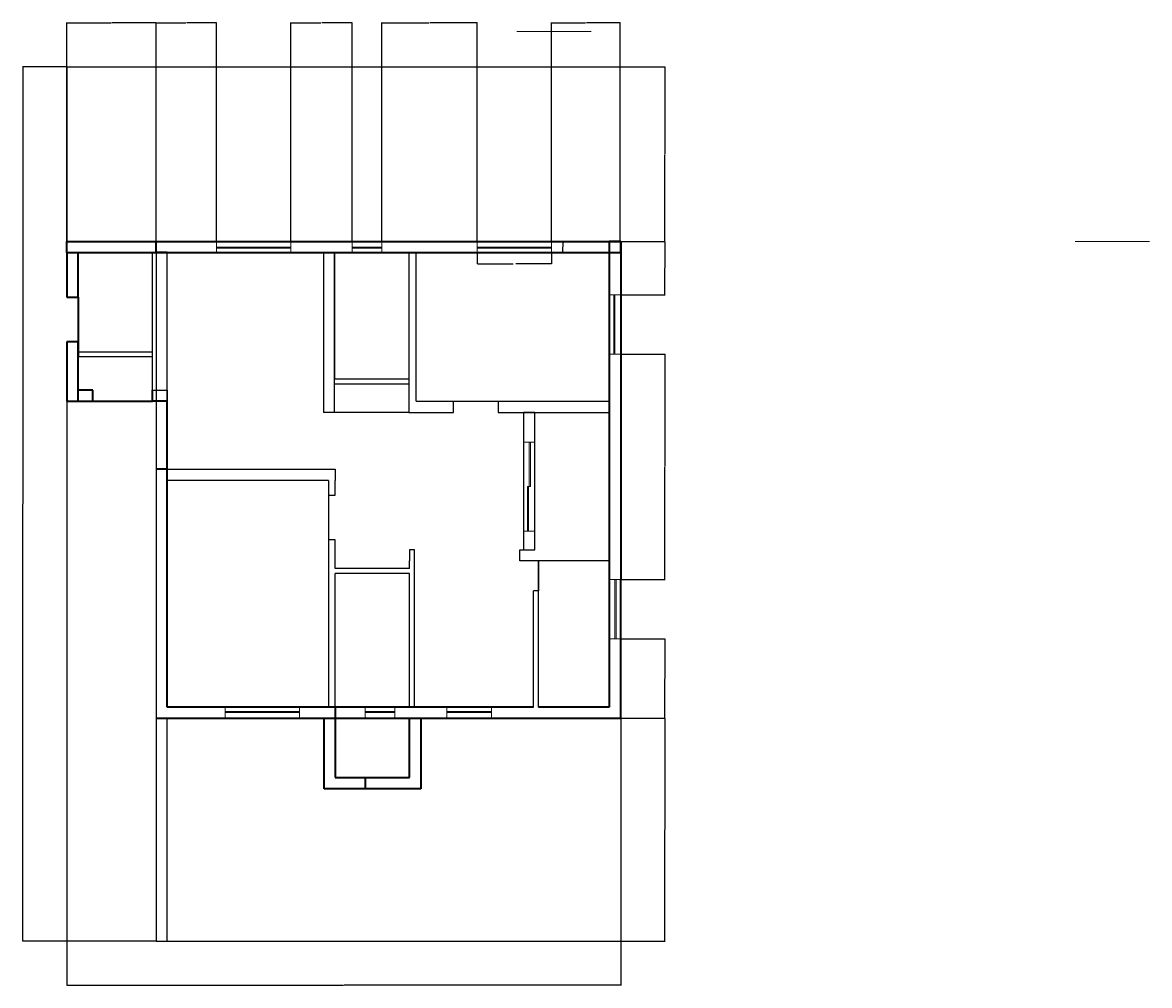
# Model space of a CAD drawing. Units: inches. Extents: x 2029 to 8798, y 1998 to 6373.
# Tile 11 of 11: x 7888 to 8798, y 1998 to 2776. Entities that reach past the tile are written whole.
import ezdxf

# ---------------------------------------------------------------- set-up
doc = ezdxf.new("R2010")
doc.units = ezdxf.units.IN
for name, color, linetype, lineweight in [('A-ANNO-DIMS', 2, 'Continuous', 18), ('A-GENM-REFR', 8, 'Continuous', 13), ('A-GLAZ', 4, 'Continuous', 18), ('A-WALL-CIRC', 7, 'Continuous', 25), ('A-WALL-EXTR', 7, 'Continuous', 35), ('A-WALL-INTR', 7, 'Continuous', 25)]:
    doc.layers.add(name, color=color, linetype=linetype, lineweight=lineweight)
doc.styles.get("Standard").update_dxf_attribs({"font": 'arial.ttf'})
doc.dimstyles.get("Standard").update_dxf_attribs({"dimtxt": 0.18, "dimasz": 0.18, "dimexe": 0.18, "dimexo": 0.0625, "dimgap": 0.09, "dimtad": 0, "dimtih": 1, "dimtoh": 1, "dimdec": 4, "dimzin": 0, "dimdsep": 46, "dimtxsty": 'Standard', "dimcen": 0.09, "dimadec": 0, "dimazin": 0, "dimtfac": 1, "dimtdec": 4, "dimtofl": 0, "dimtmove": 0, "dimatfit": 3, "dimfxl": 1, "dimtolj": 1, "dimtzin": 0, "dimarcsym": 0})

# ---------------------------------------------------------------- blocks, each defined once
blk = doc.blocks.new('WIN-60')
for p, q in [((0, 0), (0, 9)), ((0, 4.5), (60, 4.5)), ((0, 3.5), (60, 3.5)), ((60, 9), (60, 0))]:
    blk.add_line(p, q)
blk = doc.blocks.new('WIN-36')
for p, q in [((0, 36), (9, 36)), ((3.5, 36), (3.5, 0)), ((4.5, 36), (4.5, 0)), ((9, 0), (0, 0))]:
    blk.add_line(p, q)
blk = doc.blocks.new('WIN-24')
for p, q in [((0, 0), (0, 9)), ((0, 4.5), (24, 4.5)), ((0, 3.5), (24, 3.5)), ((24, 9), (24, 0))]:
    blk.add_line(p, q)
blk = doc.blocks.new('WIN-48-DEEP-JAMB')
for p, q in [((9.38, 48), (0, 48)), ((0, 48), (0, 0)), ((3.69, 48), (3.69, 0)), ((4.69, 48), (4.69, 0)), ((0, 0), (9.38, 0))]:
    blk.add_line(p, q)
blk = doc.blocks.new('GLAZ-SLIDER-72-V')
for p, q in [((0, 72), (9, 72)), ((4.5, 72), (4.5, 36)), ((5.5, 72), (5.5, 36)), ((9, 72), (9, 0)), ((3, 36), (3, 0)), ((3, 36), (4, 36)), ((4, 36), (4, 0)), ((4.5, 36), (5.5, 36)), ((9, 0), (0, 0))]:
    blk.add_line(p, q)
blk = doc.blocks.new('*D13')
at = {"layer": 'A-ANNO-DIMS', "color": 0, "lineweight": -2, "transparency": 16777216}
for p, q in [((8255.56, 2590.18), (8255.56, 2581.07)), ((8315.56, 2590.18), (8315.56, 2581.07)), ((8255.74, 2581.25), (8284.44, 2581.25)), ((8315.38, 2581.25), (8286.67, 2581.25))]:
    blk.add_line(p, q, dxfattribs=at)
at = {"layer": 'A-ANNO-DIMS', "color": 0, "transparency": 16777216}
for points in [[(8255.74, 2581.28), (8255.74, 2581.22), (8255.56, 2581.25)], [(8315.38, 2581.28), (8315.38, 2581.22), (8315.56, 2581.25)]]:
    blk.add_solid(points, dxfattribs=at)
at = {"layer": 'Defpoints', "color": 0, "transparency": 16777216}
for p in [(8255.56, 2590.25), (8315.56, 2590.25), (8315.56, 2581.25)]:
    blk.add_point(p, dxfattribs=at)
at = {"layer": 'A-ANNO-DIMS', "color": 0, "transparency": 16777216, "insert": (8285.56, 2581.25), "char_height": 0.18, "attachment_point": 5}
blk.add_mtext('\\A1;WINDOW 60 TYP.', dxfattribs=at)
blk = doc.blocks.new('*D14')
at = {"layer": 'A-ANNO-DIMS', "color": 0, "lineweight": -2, "transparency": 16777216}
for p, q in [((8315.62, 2599.25), (8324.74, 2599.25)), ((8324.56, 2599.07), (8324.56, 2594.93)), ((8324.56, 2590.43), (8324.56, 2594.57)), ((8315.62, 2590.25), (8324.74, 2590.25))]:
    blk.add_line(p, q, dxfattribs=at)
at = {"layer": 'A-ANNO-DIMS', "color": 0, "transparency": 16777216}
for points in [[(8324.53, 2599.07), (8324.59, 2599.07), (8324.56, 2599.25)], [(8324.53, 2590.43), (8324.59, 2590.43), (8324.56, 2590.25)]]:
    blk.add_solid(points, dxfattribs=at)
at = {"layer": 'Defpoints', "color": 0, "transparency": 16777216}
for p in [(8315.56, 2599.25), (8324.56, 2599.25), (8315.56, 2590.25)]:
    blk.add_point(p, dxfattribs=at)
at = {"layer": 'A-ANNO-DIMS', "color": 0, "transparency": 16777216, "insert": (8324.56, 2594.75), "char_height": 0.18, "attachment_point": 5}
blk.add_mtext('\\A1;9 TYP.', dxfattribs=at)
blk = doc.blocks.new('*D93')
at = {"layer": 'A-ANNO-DIMS', "color": 0, "lineweight": -2, "transparency": 16777216}
for p, q in [((7924.34, 2470.18), (7924.34, 1998.42)), ((8371.34, 2214.18), (8371.34, 1998.42)), ((7924.52, 1998.6), (8147.55, 1998.6)), ((8371.16, 1998.6), (8148.13, 1998.6))]:
    blk.add_line(p, q, dxfattribs=at)
at = {"layer": 'A-ANNO-DIMS', "color": 0, "transparency": 16777216}
for points in [[(7924.52, 1998.63), (7924.52, 1998.57), (7924.34, 1998.6)], [(8371.16, 1998.63), (8371.16, 1998.57), (8371.34, 1998.6)]]:
    blk.add_solid(points, dxfattribs=at)
at = {"layer": 'Defpoints', "color": 0, "transparency": 16777216}
for p in [(7924.34, 2470.25), (8371.34, 2214.25), (8371.34, 1998.6)]:
    blk.add_point(p, dxfattribs=at)
at = {"layer": 'A-ANNO-DIMS', "color": 0, "transparency": 16777216, "insert": (8147.84, 1998.6), "char_height": 0.18, "attachment_point": 5}
blk.add_mtext('\\A1;447', dxfattribs=at)
blk = doc.blocks.new('*D94')
at = {"layer": 'A-ANNO-DIMS', "color": 0, "lineweight": -2, "transparency": 16777216}
for p, q in [((7924.28, 2740.25), (7888.51, 2740.25)), ((7888.69, 2740.07), (7888.69, 2387.43)), ((7888.69, 2034.43), (7888.69, 2387.07)), ((7996.28, 2034.25), (7888.51, 2034.25))]:
    blk.add_line(p, q, dxfattribs=at)
at = {"layer": 'A-ANNO-DIMS', "color": 0, "transparency": 16777216}
for points in [[(7888.66, 2740.07), (7888.72, 2740.07), (7888.69, 2740.25)], [(7888.66, 2034.43), (7888.72, 2034.43), (7888.69, 2034.25)]]:
    blk.add_solid(points, dxfattribs=at)
at = {"layer": 'Defpoints', "color": 0, "transparency": 16777216}
for p in [(7924.34, 2740.25), (7888.69, 2034.25), (7996.34, 2034.25)]:
    blk.add_point(p, dxfattribs=at)
at = {"layer": 'A-ANNO-DIMS', "color": 0, "transparency": 16777216, "insert": (7888.69, 2387.25), "char_height": 0.18, "attachment_point": 5}
blk.add_mtext('\\A1;706', dxfattribs=at)
blk = doc.blocks.new('*D95')
at = {"layer": 'A-ANNO-DIMS', "color": 0, "lineweight": -2, "transparency": 16777216}
for p, q in [((7924.34, 2599.31), (7924.34, 2776.08)), ((7924.52, 2775.9), (7960.12, 2775.9)), ((7996.16, 2775.9), (7960.56, 2775.9)), ((7996.34, 2599.31), (7996.34, 2776.08))]:
    blk.add_line(p, q, dxfattribs=at)
at = {"layer": 'A-ANNO-DIMS', "color": 0, "transparency": 16777216}
for points in [[(7924.52, 2775.93), (7924.52, 2775.87), (7924.34, 2775.9)], [(7996.16, 2775.93), (7996.16, 2775.87), (7996.34, 2775.9)]]:
    blk.add_solid(points, dxfattribs=at)
at = {"layer": 'Defpoints', "color": 0, "transparency": 16777216}
for p in [(7996.34, 2775.9), (7924.34, 2599.25), (7996.34, 2599.25)]:
    blk.add_point(p, dxfattribs=at)
at = {"layer": 'A-ANNO-DIMS', "color": 0, "transparency": 16777216, "insert": (7960.34, 2775.9), "char_height": 0.18, "attachment_point": 5}
blk.add_mtext('\\A1;72', dxfattribs=at)
blk = doc.blocks.new('*D96')
at = {"layer": 'A-ANNO-DIMS', "color": 0, "lineweight": -2, "transparency": 16777216}
for p, q in [((7996.34, 2599.31), (7996.34, 2776.08)), ((7996.52, 2775.9), (8020.25, 2775.9)), ((8044.78, 2775.9), (8021.05, 2775.9)), ((8044.96, 2599.31), (8044.96, 2776.08))]:
    blk.add_line(p, q, dxfattribs=at)
at = {"layer": 'A-ANNO-DIMS', "color": 0, "transparency": 16777216}
for points in [[(7996.52, 2775.93), (7996.52, 2775.87), (7996.34, 2775.9)], [(8044.78, 2775.93), (8044.78, 2775.87), (8044.96, 2775.9)]]:
    blk.add_solid(points, dxfattribs=at)
at = {"layer": 'Defpoints', "color": 0, "transparency": 16777216}
for p in [(8044.96, 2775.9), (7996.34, 2599.25), (8044.96, 2599.25)]:
    blk.add_point(p, dxfattribs=at)
at = {"layer": 'A-ANNO-DIMS', "color": 0, "transparency": 16777216, "insert": (8020.65, 2775.9), "char_height": 0.18, "attachment_point": 5}
blk.add_mtext('\\A1;48.62', dxfattribs=at)
blk = doc.blocks.new('*D97')
at = {"layer": 'A-ANNO-DIMS', "color": 0, "lineweight": -2, "transparency": 16777216}
for p, q in [((8104.96, 2599.31), (8104.96, 2776.08)), ((8105.14, 2775.9), (8129.39, 2775.9)), ((8154.43, 2775.9), (8130.18, 2775.9)), ((8154.61, 2599.31), (8154.61, 2776.08))]:
    blk.add_line(p, q, dxfattribs=at)
at = {"layer": 'A-ANNO-DIMS', "color": 0, "transparency": 16777216}
for points in [[(8105.14, 2775.93), (8105.14, 2775.87), (8104.96, 2775.9)], [(8154.43, 2775.93), (8154.43, 2775.87), (8154.61, 2775.9)]]:
    blk.add_solid(points, dxfattribs=at)
at = {"layer": 'Defpoints', "color": 0, "transparency": 16777216}
for p in [(8154.61, 2775.9), (8104.96, 2599.25), (8154.61, 2599.25)]:
    blk.add_point(p, dxfattribs=at)
at = {"layer": 'A-ANNO-DIMS', "color": 0, "transparency": 16777216, "insert": (8129.78, 2775.9), "char_height": 0.18, "attachment_point": 5}
blk.add_mtext('\\A1;49.65', dxfattribs=at)
blk = doc.blocks.new('*D98')
at = {"layer": 'A-ANNO-DIMS', "color": 0, "lineweight": -2, "transparency": 16777216}
for p, q in [((8178.61, 2599.31), (8178.61, 2776.08)), ((8178.79, 2775.9), (8216.69, 2775.9)), ((8255.38, 2775.9), (8217.48, 2775.9)), ((8255.56, 2599.31), (8255.56, 2776.08))]:
    blk.add_line(p, q, dxfattribs=at)
at = {"layer": 'A-ANNO-DIMS', "color": 0, "transparency": 16777216}
for points in [[(8178.79, 2775.93), (8178.79, 2775.87), (8178.61, 2775.9)], [(8255.38, 2775.93), (8255.38, 2775.87), (8255.56, 2775.9)]]:
    blk.add_solid(points, dxfattribs=at)
at = {"layer": 'Defpoints', "color": 0, "transparency": 16777216}
for p in [(8255.56, 2775.9), (8178.61, 2599.25), (8255.56, 2599.25)]:
    blk.add_point(p, dxfattribs=at)
at = {"layer": 'A-ANNO-DIMS', "color": 0, "transparency": 16777216, "insert": (8217.08, 2775.9), "char_height": 0.18, "attachment_point": 5}
blk.add_mtext('\\A1;76.95', dxfattribs=at)
blk = doc.blocks.new('*D99')
at = {"layer": 'A-ANNO-DIMS', "color": 0, "lineweight": -2, "transparency": 16777216}
for p, q in [((8315.56, 2599.31), (8315.56, 2776.08)), ((8315.74, 2775.9), (8342.88, 2775.9)), ((8370.78, 2775.9), (8343.64, 2775.9)), ((8370.96, 2599.31), (8370.96, 2776.08))]:
    blk.add_line(p, q, dxfattribs=at)
at = {"layer": 'A-ANNO-DIMS', "color": 0, "transparency": 16777216}
for points in [[(8315.74, 2775.93), (8315.74, 2775.87), (8315.56, 2775.9)], [(8370.78, 2775.93), (8370.78, 2775.87), (8370.96, 2775.9)]]:
    blk.add_solid(points, dxfattribs=at)
at = {"layer": 'Defpoints', "color": 0, "transparency": 16777216}
for p in [(8370.96, 2775.9), (8315.56, 2599.25), (8370.96, 2599.25)]:
    blk.add_point(p, dxfattribs=at)
at = {"layer": 'A-ANNO-DIMS', "color": 0, "transparency": 16777216, "insert": (8343.26, 2775.9), "char_height": 0.18, "attachment_point": 5}
blk.add_mtext('\\A1;55.41', dxfattribs=at)
blk = doc.blocks.new('*D100')
at = {"layer": 'A-ANNO-DIMS', "color": 0, "lineweight": -2, "transparency": 16777216}
for p, q in [((8371.4, 2214.25), (8407.17, 2214.25)), ((8406.99, 2214.07), (8406.99, 2124.43)), ((8406.99, 2034.43), (8406.99, 2124.07)), ((7996.4, 2034.25), (8407.17, 2034.25))]:
    blk.add_line(p, q, dxfattribs=at)
at = {"layer": 'A-ANNO-DIMS', "color": 0, "transparency": 16777216}
for points in [[(8406.96, 2214.07), (8407.02, 2214.07), (8406.99, 2214.25)], [(8406.96, 2034.43), (8407.02, 2034.43), (8406.99, 2034.25)]]:
    blk.add_solid(points, dxfattribs=at)
at = {"layer": 'Defpoints', "color": 0, "transparency": 16777216}
for p in [(8371.34, 2214.25), (8406.99, 2214.25), (7996.34, 2034.25)]:
    blk.add_point(p, dxfattribs=at)
at = {"layer": 'A-ANNO-DIMS', "color": 0, "transparency": 16777216, "insert": (8406.99, 2124.25), "char_height": 0.18, "attachment_point": 5}
blk.add_mtext('\\A1;180', dxfattribs=at)
blk = doc.blocks.new('*D101')
at = {"layer": 'A-ANNO-DIMS', "color": 0, "lineweight": -2, "transparency": 16777216}
for p, q in [((8371.4, 2278.25), (8407.17, 2278.25)), ((8406.99, 2278.07), (8406.99, 2246.43)), ((8406.99, 2214.43), (8406.99, 2246.07)), ((8371.4, 2214.25), (8407.17, 2214.25))]:
    blk.add_line(p, q, dxfattribs=at)
at = {"layer": 'A-ANNO-DIMS', "color": 0, "transparency": 16777216}
for points in [[(8406.96, 2278.07), (8407.02, 2278.07), (8406.99, 2278.25)], [(8406.96, 2214.43), (8407.02, 2214.43), (8406.99, 2214.25)]]:
    blk.add_solid(points, dxfattribs=at)
at = {"layer": 'Defpoints', "color": 0, "transparency": 16777216}
for p in [(8371.34, 2278.25), (8406.99, 2278.25), (8371.34, 2214.25)]:
    blk.add_point(p, dxfattribs=at)
at = {"layer": 'A-ANNO-DIMS', "color": 0, "transparency": 16777216, "insert": (8406.99, 2246.25), "char_height": 0.18, "attachment_point": 5}
blk.add_mtext('\\A1;64', dxfattribs=at)
blk = doc.blocks.new('*D102')
at = {"layer": 'A-ANNO-DIMS', "color": 0, "lineweight": -2, "transparency": 16777216}
for p, q in [((8371.4, 2508.3), (8407.17, 2508.3)), ((8406.99, 2508.12), (8406.99, 2417.45)), ((8406.99, 2326.43), (8406.99, 2417.09)), ((8371.4, 2326.25), (8407.17, 2326.25))]:
    blk.add_line(p, q, dxfattribs=at)
at = {"layer": 'A-ANNO-DIMS', "color": 0, "transparency": 16777216}
for points in [[(8406.96, 2508.12), (8407.02, 2508.12), (8406.99, 2508.3)], [(8406.96, 2326.43), (8407.02, 2326.43), (8406.99, 2326.25)]]:
    blk.add_solid(points, dxfattribs=at)
at = {"layer": 'Defpoints', "color": 0, "transparency": 16777216}
for p in [(8371.34, 2508.3), (8406.99, 2508.3), (8371.34, 2326.25)]:
    blk.add_point(p, dxfattribs=at)
at = {"layer": 'A-ANNO-DIMS', "color": 0, "transparency": 16777216, "insert": (8406.99, 2417.27), "char_height": 0.18, "attachment_point": 5}
blk.add_mtext('\\A1;182.05', dxfattribs=at)
blk = doc.blocks.new('*D103')
at = {"layer": 'A-ANNO-DIMS', "color": 0, "lineweight": -2, "transparency": 16777216}
for p, q in [((8371.03, 2599.25), (8407.17, 2599.25)), ((8406.99, 2599.07), (8406.99, 2577.95)), ((8406.99, 2556.48), (8406.99, 2577.59)), ((8371.4, 2556.3), (8407.17, 2556.3))]:
    blk.add_line(p, q, dxfattribs=at)
at = {"layer": 'A-ANNO-DIMS', "color": 0, "transparency": 16777216}
for points in [[(8406.96, 2599.07), (8407.02, 2599.07), (8406.99, 2599.25)], [(8406.96, 2556.48), (8407.02, 2556.48), (8406.99, 2556.3)]]:
    blk.add_solid(points, dxfattribs=at)
at = {"layer": 'Defpoints', "color": 0, "transparency": 16777216}
for p in [(8370.96, 2599.25), (8406.99, 2599.25), (8371.34, 2556.3)]:
    blk.add_point(p, dxfattribs=at)
at = {"layer": 'A-ANNO-DIMS', "color": 0, "transparency": 16777216, "insert": (8406.99, 2577.77), "char_height": 0.18, "attachment_point": 5}
blk.add_mtext('\\A1;42.95', dxfattribs=at)
blk = doc.blocks.new('*D104')
at = {"layer": 'A-ANNO-DIMS', "color": 0, "lineweight": -2, "transparency": 16777216}
for p, q in [((7924.4, 2740.25), (8407.17, 2740.25)), ((8406.99, 2740.07), (8406.99, 2669.93)), ((8406.99, 2599.43), (8406.99, 2669.57)), ((7924.4, 2599.25), (8407.17, 2599.25))]:
    blk.add_line(p, q, dxfattribs=at)
at = {"layer": 'A-ANNO-DIMS', "color": 0, "transparency": 16777216}
for points in [[(8406.96, 2740.07), (8407.02, 2740.07), (8406.99, 2740.25)], [(8406.96, 2599.43), (8407.02, 2599.43), (8406.99, 2599.25)]]:
    blk.add_solid(points, dxfattribs=at)
at = {"layer": 'Defpoints', "color": 0, "transparency": 16777216}
for p in [(7924.34, 2740.25), (8406.99, 2740.25), (7924.34, 2599.25)]:
    blk.add_point(p, dxfattribs=at)
at = {"layer": 'A-ANNO-DIMS', "color": 0, "transparency": 16777216, "insert": (8406.99, 2669.75), "char_height": 0.18, "attachment_point": 5}
blk.add_mtext('\\A1;141', dxfattribs=at)

msp = doc.modelspace()

# ---------------------------------------------------------------- linework, layer by layer
at = {"layer": 'A-GENM-REFR'}
for p, q in [((8287.3629, 2768.7471), (8347.3629, 2768.7471)), ((8738.1455, 2599.2471), (8798.1455, 2599.2471))]:
    msp.add_line(p, q, dxfattribs=at)
at = {"layer": 'A-GLAZ'}
for p, q in [((8044.9596, 2599.2471), (8104.9596, 2599.2471)), ((8154.6092, 2599.2471), (8178.6092, 2599.2471)), ((8255.5559, 2599.2471), (8315.5559, 2599.2471)), ((8112.0384, 2214.2471), (8052.0384, 2214.2471)), ((8188.9632, 2214.2471), (8164.9632, 2214.2471)), ((8267.1078, 2214.2471), (8231.1078, 2214.2471))]:
    msp.add_line(p, q, dxfattribs=at)
at = {"layer": 'A-WALL-CIRC'}
for p, q in [((7924.342, 2740.2471), (7924.342, 2590.2471)), ((7996.342, 2214.2471), (7996.342, 2094.2471)), ((8005.342, 2034.2471), (8005.342, 2214.2471)), ((7996.342, 2094.2471), (7996.342, 2034.2471)), ((7996.342, 2034.2471), (8005.342, 2034.2471))]:
    msp.add_line(p, q, dxfattribs=at)
at = {"layer": 'A-WALL-EXTR'}
for p, q in [((7924.342, 2590.2471), (7924.342, 2599.2471)), ((7924.342, 2599.2471), (8370.9632, 2599.2471)), ((7996.342, 2590.2471), (7996.342, 2599.2471)), ((8370.9632, 2599.2471), (8361.9632, 2599.2471)), ((8361.9632, 2599.2471), (8361.9632, 2326.2471)), ((8371.342, 2599.2471), (8369.0749, 2599.2471)), ((8371.342, 2590.2471), (8371.342, 2599.2471)), ((8371.342, 2599.2471), (8371.342, 2326.2471)), ((7924.342, 2590.2471), (7924.342, 2554.2471)), ((7924.342, 2590.2471), (8131.342, 2590.2471)), ((7933.342, 2554.2471), (7933.342, 2590.2471)), ((8005.342, 2590.2471), (7996.342, 2590.2471)), ((8005.342, 2590.2471), (8131.342, 2590.2471)), ((8005.342, 2590.2471), (8044.9596, 2590.2471)), ((8027.842, 2590.2471), (8133.7725, 2590.2471)), ((8131.342, 2590.2471), (8371.342, 2590.2471)), ((8140.342, 2590.2471), (8200.342, 2590.2471)), ((8140.342, 2590.2471), (8154.6092, 2590.2471)), ((8206.342, 2590.2471), (8255.5559, 2590.2471)), ((8371.342, 2590.2471), (8371.342, 2556.2967)), ((7924.342, 2554.2471), (7933.342, 2554.2471)), ((7933.342, 2554.2471), (7933.342, 2518.2471)), ((7933.342, 2518.2471), (7924.342, 2518.2471)), ((7924.342, 2518.2471), (7924.342, 2470.2471)), ((7933.342, 2470.2471), (7933.342, 2518.2471)), ((7933.342, 2518.2471), (7933.342, 2506.2471)), ((7945.342, 2479.2471), (7933.342, 2479.2471)), ((7945.342, 2470.2471), (7945.342, 2479.2471)), ((7993.342, 2470.2471), (7993.342, 2479.2471)), ((7924.342, 2470.2471), (7933.342, 2470.2471)), ((7933.342, 2470.2471), (7945.342, 2470.2471)), ((7945.342, 2470.2471), (7993.342, 2470.2471)), ((8005.342, 2470.2471), (7993.342, 2470.2471)), ((8005.342, 2470.2471), (7993.342, 2470.2471)), ((8005.342, 2223.2471), (8005.342, 2470.2471)), ((8361.9632, 2461.2471), (8361.9632, 2341.2471)), ((8005.342, 2415.2471), (7996.342, 2415.2471)), ((8005.342, 2415.2471), (8005.342, 2415.2471)), ((8005.342, 2406.2471), (8005.342, 2415.2471)), ((8005.342, 2223.2471), (8005.342, 2406.2471)), ((8361.9632, 2341.2471), (8361.9632, 2223.2471)), ((8371.342, 2223.2471), (8371.342, 2326.2471)), ((8298.9632, 2223.2471), (8005.342, 2223.2471)), ((8135.342, 2223.2471), (8112.0384, 2223.2471)), ((8196.9632, 2223.2471), (8136.9632, 2223.2471)), ((8200.9632, 2223.2471), (8140.9632, 2223.2471)), ((8200.9632, 2223.2471), (8140.9632, 2223.2471)), ((8140.9632, 2223.2471), (8140.9632, 2214.2471)), ((8200.9632, 2223.2471), (8188.9632, 2223.2471)), ((8298.9632, 2223.2471), (8202.9632, 2223.2471)), ((8298.9632, 2223.2471), (8267.1078, 2223.2471)), ((8300.9632, 2223.2471), (8298.9632, 2223.2471)), ((8361.9632, 2223.2471), (8304.9632, 2223.2471)), ((8361.9632, 2223.2471), (8304.9632, 2223.2471)), ((8371.342, 2214.2471), (8371.342, 2223.2471)), ((7996.342, 2214.2471), (8371.342, 2214.2471)), ((8131.9632, 2157.2471), (8131.9632, 2214.2471)), ((8140.9632, 2214.2471), (8140.9632, 2166.2471)), ((8200.9632, 2166.2471), (8200.9632, 2214.2471)), ((8200.9632, 2214.2471), (8209.9632, 2214.2471)), ((8209.9632, 2214.2471), (8209.9632, 2157.2471)), ((8140.9632, 2166.2471), (8164.9632, 2166.2471)), ((8164.9632, 2166.2471), (8164.9632, 2157.2471)), ((8164.9632, 2166.2471), (8200.9632, 2166.2471)), ((8140.9632, 2157.2471), (8131.9632, 2157.2471)), ((8164.9632, 2157.2471), (8140.9632, 2157.2471)), ((8209.9632, 2157.2471), (8164.9632, 2157.2471))]:
    msp.add_line(p, q, dxfattribs=at)
at = {"layer": 'A-WALL-INTR'}
for p, q in [((7993.342, 2479.2471), (7993.342, 2590.2471)), ((7996.342, 2590.2471), (7996.342, 2214.2471)), ((8005.342, 2470.2471), (8005.342, 2590.2471)), ((8131.342, 2590.2471), (8131.342, 2461.2471)), ((8140.342, 2461.2471), (8140.342, 2590.2471)), ((8140.342, 2590.2471), (8140.342, 2488.2471)), ((8200.342, 2590.2471), (8200.342, 2470.2471)), ((8206.342, 2470.2471), (8206.342, 2590.2471)), ((7933.342, 2510.2471), (7993.342, 2510.2471)), ((7933.342, 2506.2471), (7993.342, 2506.2471)), ((8140.342, 2488.2471), (8200.342, 2488.2471)), ((8140.342, 2484.2471), (8200.342, 2484.2471)), ((7993.342, 2479.2471), (8005.342, 2479.2471)), ((8005.342, 2479.2471), (8005.342, 2470.2471)), ((8200.342, 2470.2471), (8200.342, 2461.2471)), ((8206.342, 2470.2471), (8361.9632, 2470.2471)), ((8236.342, 2461.2471), (8236.342, 2470.2471)), ((8236.342, 2470.2471), (8272.342, 2470.2471)), ((8272.342, 2470.2471), (8272.342, 2461.2471)), ((8140.342, 2461.2471), (8131.342, 2461.2471)), ((8200.342, 2461.2471), (8140.342, 2461.2471)), ((8200.342, 2461.2471), (8206.342, 2461.2471)), ((8200.342, 2461.2471), (8236.342, 2461.2471)), ((8206.342, 2461.2471), (8236.342, 2461.2471)), ((8272.342, 2461.2471), (8361.9632, 2461.2471)), ((8301.9632, 2461.2471), (8292.9632, 2461.2471)), ((8292.9632, 2461.2471), (8292.9632, 2350.2471)), ((8292.9632, 2461.2471), (8292.9632, 2437.2471)), ((8301.9632, 2350.2471), (8301.9632, 2461.2471)), ((8005.342, 2415.2471), (8140.9632, 2415.2471)), ((8140.9632, 2415.2471), (8140.9632, 2406.2471)), ((8135.342, 2406.2471), (8005.342, 2406.2471)), ((8135.342, 2406.2471), (8135.342, 2223.2471)), ((8135.342, 2406.2471), (8135.342, 2394.2471)), ((8140.9632, 2394.2471), (8140.9632, 2406.2471)), ((8135.342, 2394.2471), (8140.9632, 2394.2471)), ((8140.9632, 2358.2471), (8135.342, 2358.2471)), ((8140.9632, 2335.2471), (8140.9632, 2358.2471)), ((8204.9632, 2350.2471), (8200.9632, 2350.2471)), ((8200.9632, 2350.2471), (8200.9632, 2341.2471)), ((8204.9632, 2341.2471), (8204.9632, 2350.2471)), ((8289.9632, 2341.2471), (8289.9632, 2350.2471)), ((8289.9632, 2350.2471), (8301.9632, 2350.2471)), ((8200.9632, 2335.2471), (8200.9632, 2341.2471)), ((8204.9632, 2223.2471), (8204.9632, 2341.2471)), ((8361.9632, 2341.2471), (8289.9632, 2341.2471)), ((8304.9632, 2341.2471), (8300.9632, 2341.2471)), ((8304.9632, 2223.2471), (8304.9632, 2341.2471)), ((8304.9632, 2341.2471), (8304.9632, 2317.2471)), ((8200.9632, 2335.2471), (8140.9632, 2335.2471)), ((8140.9632, 2223.2471), (8140.9632, 2331.2471)), ((8200.9632, 2331.2471), (8140.9632, 2331.2471)), ((8200.9632, 2223.2471), (8200.9632, 2331.2471)), ((8200.9632, 2223.2471), (8200.9632, 2331.2471)), ((8300.9632, 2223.2471), (8300.9632, 2317.2471)), ((8304.9632, 2317.2471), (8300.9632, 2317.2471))]:
    msp.add_line(p, q, dxfattribs=at)

# ---------------------------------------------------------------- block references
at = {"layer": 'A-GLAZ'}
for name, p in [('WIN-60', (8044.9596, 2590.2471)), ('WIN-24', (8154.6092, 2590.2471)), ('WIN-60', (8255.5559, 2590.2471)), ('WIN-48-DEEP-JAMB', (8361.9632, 2508.2967)), ('GLAZ-SLIDER-72-V', (8292.9632, 2365.2471))]:
    msp.add_blockref(name, p, dxfattribs=at)
at = {"layer": 'A-GLAZ', "extrusion": (0, 0, -1), "zscale": -1}
msp.add_blockref('WIN-48-DEEP-JAMB', (-8371.342, 2278.2471), dxfattribs=at)
at = {"layer": 'A-GLAZ', "extrusion": (0, 0, -1), "zscale": -1, "rotation": 180}
for name, p in [('WIN-60', (-8052.0384, 2223.2471)), ('WIN-24', (-8164.9632, 2223.2471))]:
    msp.add_blockref(name, p, dxfattribs=at)
at = {"layer": 'A-GLAZ', "rotation": 270}
msp.add_blockref('WIN-36', (8231.1078, 2223.2471), dxfattribs=at)

# ---------------------------------------------------------------- dimensions: what is measured, and where the dimension line sits
at = {"layer": 'A-ANNO-DIMS'}
for base, p1, p2, override, picture, middle in [((7996.342, 2775.8971), (7924.342, 2599.2471), (7996.342, 2599.2471), {"dimdec": 0, "dimlfac": 1, "dimrnd": 0, "dimzin": 0, "dimdsep": 46, "dimlunit": 2}, '*D95', (7960.342, 2775.8971)), ((8044.9596, 2775.8971), (7996.342, 2599.2471), (8044.9596, 2599.2471), {"dimdec": 2, "dimlfac": 1, "dimrnd": 0, "dimzin": 0, "dimdsep": 46, "dimlunit": 2}, '*D96', (8020.6508, 2775.8971)), ((8154.6092, 2775.8971), (8104.9596, 2599.2471), (8154.6092, 2599.2471), {"dimdec": 2, "dimlfac": 1, "dimrnd": 0, "dimzin": 0, "dimdsep": 46, "dimlunit": 2}, '*D97', (8129.7844, 2775.8971)), ((8255.5559, 2775.8971), (8178.6092, 2599.2471), (8255.5559, 2599.2471), {"dimdec": 2, "dimlfac": 1, "dimrnd": 0, "dimzin": 0, "dimdsep": 46, "dimlunit": 2}, '*D98', (8217.0825, 2775.8971)), ((8370.9632, 2775.8971), (8315.5559, 2599.2471), (8370.9632, 2599.2471), {"dimdec": 2, "dimlfac": 1, "dimrnd": 0, "dimzin": 0, "dimdsep": 46, "dimlunit": 2}, '*D99', (8343.2595, 2775.8971)), ((8371.342, 1998.5971), (7924.342, 2470.2471), (8371.342, 2214.2471), {"dimdec": 0, "dimlfac": 1, "dimrnd": 0, "dimzin": 0, "dimdsep": 46, "dimlunit": 2}, '*D93', (8147.842, 1998.5971))]:
    dim = msp.add_linear_dim(base=base, p1=p1, p2=p2, dimstyle='Standard', override=override, dxfattribs=at)
    dim.commit()
    dim.dimension.update_dxf_attribs({"geometry": picture, "text_midpoint": middle})
for base, p1, p2, override, picture, middle in [((7888.692, 2034.2471), (7924.342, 2740.2471), (7996.342, 2034.2471), {"dimdec": 0, "dimlfac": 1, "dimrnd": 0, "dimzin": 0, "dimdsep": 46, "dimlunit": 2}, '*D94', (7888.692, 2387.2471)), ((8406.992, 2740.2471), (7924.342, 2599.2471), (7924.342, 2740.2471), {"dimdec": 0, "dimlfac": 1, "dimrnd": 0, "dimzin": 0, "dimdsep": 46, "dimlunit": 2}, '*D104', (8406.992, 2669.7471)), ((8406.992, 2599.2471), (8371.342, 2556.2967), (8370.9632, 2599.2471), {"dimdec": 2, "dimlfac": 1, "dimrnd": 0, "dimzin": 0, "dimdsep": 46, "dimlunit": 2}, '*D103', (8406.992, 2577.7719)), ((8406.992, 2508.2967), (8371.342, 2326.2471), (8371.342, 2508.2967), {"dimdec": 2, "dimlfac": 1, "dimrnd": 0, "dimzin": 0, "dimdsep": 46, "dimlunit": 2}, '*D102', (8406.992, 2417.2719)), ((8406.992, 2278.2471), (8371.342, 2214.2471), (8371.342, 2278.2471), {"dimdec": 0, "dimlfac": 1, "dimrnd": 0, "dimzin": 0, "dimdsep": 46, "dimlunit": 2}, '*D101', (8406.992, 2246.2471)), ((8406.992, 2214.2471), (7996.342, 2034.2471), (8371.342, 2214.2471), {"dimdec": 0, "dimlfac": 1, "dimrnd": 0, "dimzin": 0, "dimdsep": 46, "dimlunit": 2}, '*D100', (8406.992, 2124.2471))]:
    dim = msp.add_linear_dim(base=base, p1=p1, p2=p2, angle=90, dimstyle='Standard', override=override, dxfattribs=at)
    dim.commit()
    dim.dimension.update_dxf_attribs({"geometry": picture, "text_midpoint": middle})
dim = msp.add_linear_dim(base=(8324.5559, 2599.2471), p1=(8315.5559, 2590.2471), p2=(8315.5559, 2599.2471), angle=90, text='<> TYP.', dimstyle='Standard', override={"dimdec": 0, "dimlfac": 1, "dimrnd": 0, "dimzin": 0, "dimdsep": 46, "dimlunit": 2}, dxfattribs=at)
dim.commit()
dim.dimension.update_dxf_attribs({"geometry": '*D14', "text_midpoint": (8324.5559, 2594.7471)})
dim = msp.add_linear_dim(base=(8315.5559, 2581.2471), p1=(8255.5559, 2590.2471), p2=(8315.5559, 2590.2471), text='WINDOW <> TYP.', dimstyle='Standard', override={"dimdec": 0, "dimlfac": 1, "dimrnd": 0, "dimzin": 0, "dimdsep": 46, "dimlunit": 2}, dxfattribs=at)
dim.commit()
dim.dimension.update_dxf_attribs({"geometry": '*D13', "text_midpoint": (8285.5559, 2581.2471)})

doc.saveas('drawing.dxf')
